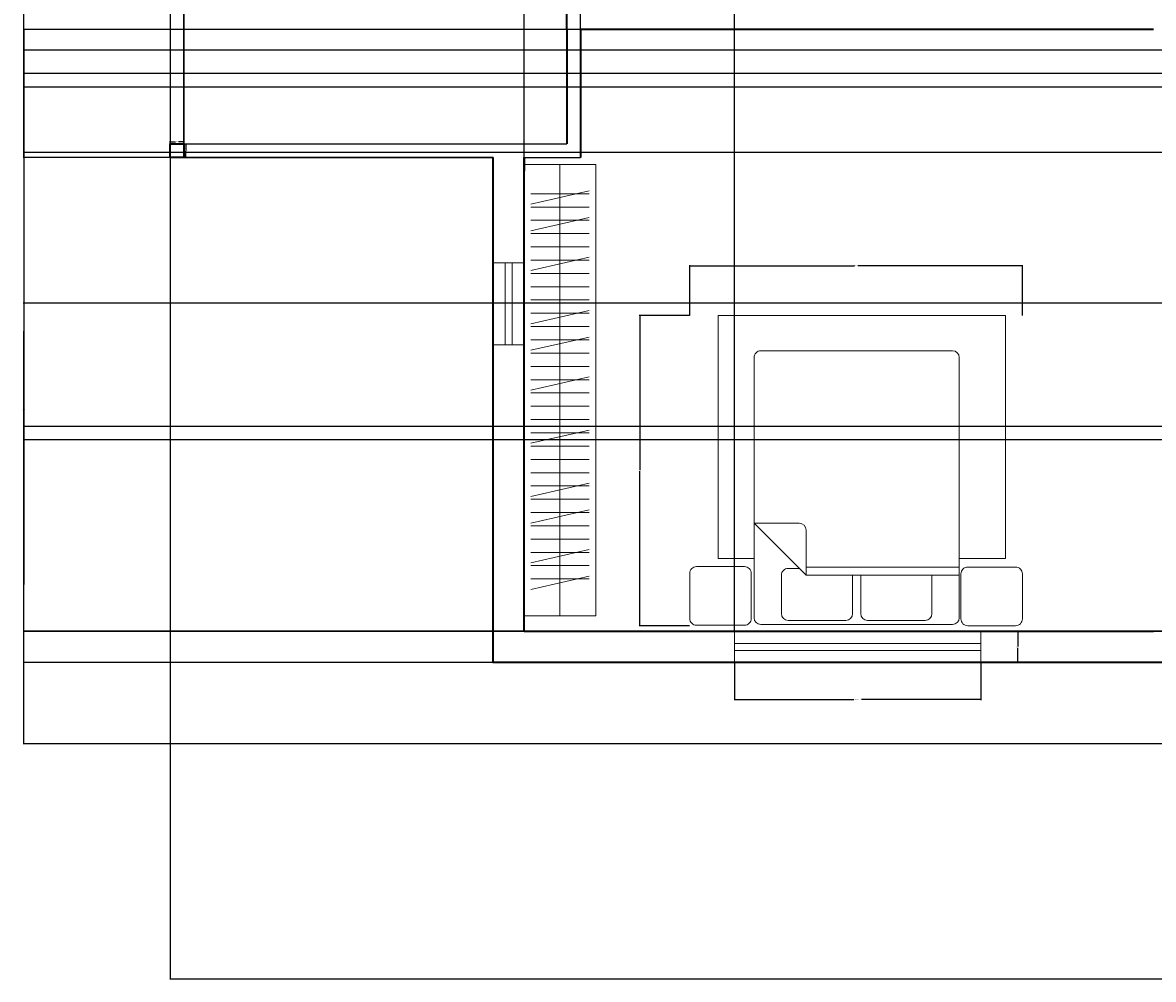
# Model space of a CAD drawing. Units: inches. Extents: x 2024 to 2965, y 1692 to 2308.
# Tile 1 of 8: x 2024 to 2355, y 1692 to 1972. Entities that reach past the tile are written whole.
import ezdxf

# ---------------------------------------------------------------- set-up
doc = ezdxf.new("R2010")
doc.units = ezdxf.units.IN
for name, color, linetype, lineweight in [('A-ANNO-DIMS', 2, 'Continuous', 18), ('A-COLS', 1, 'Continuous', 35), ('A-FLOR-CASE', 33, 'Continuous', 20), ('A-FLOR-CASE-PATT', 252, 'Continuous', 13), ('A-FLOR-OTLN', 7, 'Continuous', 25), ('A-FURN', 8, 'Continuous', 18), ('A-GLAZ', 4, 'Continuous', 18), ('A-WALL', 7, 'Continuous', 35)]:
    doc.layers.add(name, color=color, linetype=linetype, lineweight=lineweight)
doc.styles.get("Standard").update_dxf_attribs({"font": 'arial.ttf'})
doc.dimstyles.get("Standard").update_dxf_attribs({"dimtxt": 0.18, "dimasz": 0.18, "dimexe": 0.18, "dimexo": 0.0625, "dimgap": 0.09, "dimtad": 0, "dimtih": 1, "dimtoh": 1, "dimdec": 4, "dimzin": 0, "dimdsep": 46, "dimtxsty": 'Standard', "dimcen": 0.09, "dimadec": 0, "dimazin": 0, "dimtfac": 1, "dimtdec": 4, "dimtofl": 0, "dimtmove": 0, "dimatfit": 3, "dimfxl": 1, "dimtolj": 1, "dimtzin": 0, "dimarcsym": 0})

# ---------------------------------------------------------------- blocks, each defined once
blk = doc.blocks.new('Bed - Queen')
for p, q in [((2, 0), (58, 0)), ((0, -78), (0, -2)), ((8, -14.4), (8, -3.2)), ((10, -1.2), (26.8, -1.2)), ((28.8, -3.2), (28.8, -14.4)), ((31.2, -14.4), (31.2, -3.2)), ((33.2, -1.2), (50, -1.2)), ((52, -3.2), (52, -14.4)), ((60, -2), (60, -78)), ((0, -14.4), (44.8, -14.4)), ((60, -29.6), (44.8, -14.4)), ((44.8, -14.4), (44.8, -27.6)), ((50, -16.4), (46.8, -16.4)), ((44.8, -16.8), (0, -16.8)), ((46.8, -29.6), (60, -29.6)), ((58, -80), (2, -80))]:
    blk.add_line(p, q)
for points in [[(-16.47, 0.34), (-2.47, 0.34, -0.414214), (-0.47, -1.66), (-0.47, -14.8, -0.414214), (-2.47, -16.8), (-16.47, -16.8, -0.414214), (-18.47, -14.8), (-18.47, -1.66, -0.414214)], [(62.82, 0.21), (76.82, 0.21, -0.414214), (78.82, -1.79), (78.82, -14.93, -0.414214), (76.82, -16.93), (62.82, -16.93, -0.414214), (60.82, -14.93), (60.82, -1.79, -0.414214)]]:
    blk.add_lwpolyline(points, format="xyb", close=True)
blk.add_lwpolyline([(0, -19.29), (-13.55, -19.29), (-13.55, -90.28), (70.45, -90.28), (70.45, -19.29), (60, -19.29)])
for centre, start, end in [((2, -2), 90, 180), ((58, -2), 0, 90), ((10, -3.2), 90, 180), ((26.8, -3.2), 0, 90), ((33.2, -3.2), 90, 180), ((50, -3.2), 0, 90), ((50, -14.4), 270, 0), ((46.8, -27.6), 180, 270), ((2, -78), 180, 270), ((58, -78), 270, 0)]:
    blk.add_arc(centre, 2, start, end)
blk = doc.blocks.new('WIN-24-D9')
for p, q in [((0, 5.5), (24, 5.5)), ((0, 3.5), (24, 3.5))]:
    blk.add_line(p, q)
for points in [[(0, 0), (0, 9)], [(24, 9), (24, 0)]]:
    blk.add_lwpolyline(points)
blk = doc.blocks.new('WIN-72-D9')
for p, q in [((0, 5.5), (72, 5.5)), ((0, 3.5), (72, 3.5))]:
    blk.add_line(p, q)
for points in [[(0, 0), (0, 9)], [(72, 9), (72, 0)]]:
    blk.add_lwpolyline(points)
blk = doc.blocks.new('POST-4X4')
blk.add_lwpolyline([(0, 4), (4, 4), (4, 0), (0, 0)], close=True)
blk = doc.blocks.new('*D33')
at = {"layer": 'A-ANNO-DIMS', "color": 0, "lineweight": -2, "transparency": 16777216}
for p, q in [((2232.43, 1784.71), (2232.43, 1773.79)), ((2304.43, 1784.71), (2304.43, 1773.79)), ((2232.61, 1773.97), (2267.31, 1773.97)), ((2304.25, 1773.97), (2269.55, 1773.97))]:
    blk.add_line(p, q, dxfattribs=at)
at = {"layer": 'A-ANNO-DIMS', "color": 0, "transparency": 16777216}
for points in [[(2232.61, 1774), (2232.61, 1773.94), (2232.43, 1773.97)], [(2304.25, 1774), (2304.25, 1773.94), (2304.43, 1773.97)]]:
    blk.add_solid(points, dxfattribs=at)
at = {"layer": 'Defpoints', "color": 0, "transparency": 16777216}
for p in [(2232.43, 1784.77), (2304.43, 1784.77), (2304.43, 1773.97)]:
    blk.add_point(p, dxfattribs=at)
at = {"layer": 'A-ANNO-DIMS', "color": 0, "transparency": 16777216, "insert": (2268.43, 1773.97), "char_height": 0.18, "attachment_point": 5}
blk.add_mtext('\\A1;WINDOW 72 TYP.', dxfattribs=at)
blk = doc.blocks.new('*D34')
at = {"layer": 'A-ANNO-DIMS', "color": 0, "lineweight": -2, "transparency": 16777216}
for p, q in [((2304.49, 1793.77), (2315.41, 1793.77)), ((2315.23, 1793.59), (2315.23, 1789.46)), ((2315.23, 1784.95), (2315.23, 1789.09)), ((2304.49, 1784.77), (2315.41, 1784.77))]:
    blk.add_line(p, q, dxfattribs=at)
at = {"layer": 'A-ANNO-DIMS', "color": 0, "transparency": 16777216}
for points in [[(2315.2, 1793.59), (2315.26, 1793.59), (2315.23, 1793.77)], [(2315.2, 1784.95), (2315.26, 1784.95), (2315.23, 1784.77)]]:
    blk.add_solid(points, dxfattribs=at)
at = {"layer": 'Defpoints', "color": 0, "transparency": 16777216}
for p in [(2304.43, 1793.77), (2315.23, 1793.77), (2304.43, 1784.77)]:
    blk.add_point(p, dxfattribs=at)
at = {"layer": 'A-ANNO-DIMS', "color": 0, "transparency": 16777216, "insert": (2315.23, 1789.27), "char_height": 0.18, "attachment_point": 5}
blk.add_mtext('\\A1;9 TYP.', dxfattribs=at)
blk = doc.blocks.new('*D45')
at = {"layer": 'A-ANNO-DIMS', "color": 0, "lineweight": -2, "transparency": 16777216}
for p, q in [((2219.34, 1886.2), (2219.34, 1900.91)), ((2219.52, 1900.73), (2267.48, 1900.73)), ((2316.45, 1900.73), (2268.49, 1900.73)), ((2316.63, 1886.2), (2316.63, 1900.91))]:
    blk.add_line(p, q, dxfattribs=at)
at = {"layer": 'A-ANNO-DIMS', "color": 0, "transparency": 16777216}
for points in [[(2219.52, 1900.76), (2219.52, 1900.7), (2219.34, 1900.73)], [(2316.45, 1900.76), (2316.45, 1900.7), (2316.63, 1900.73)]]:
    blk.add_solid(points, dxfattribs=at)
at = {"layer": 'Defpoints', "color": 0, "transparency": 16777216}
for p in [(2219.34, 1900.73), (2219.34, 1886.14), (2316.63, 1886.14)]:
    blk.add_point(p, dxfattribs=at)
at = {"layer": 'A-ANNO-DIMS', "color": 0, "transparency": 16777216, "insert": (2267.99, 1900.73), "char_height": 0.18, "attachment_point": 5}
blk.add_mtext('\\A1;BED 97', dxfattribs=at)
blk = doc.blocks.new('*D46')
at = {"layer": 'A-ANNO-DIMS', "color": 0, "lineweight": -2, "transparency": 16777216}
for p, q in [((2219.27, 1886.14), (2204.56, 1886.14)), ((2204.74, 1885.96), (2204.74, 1841.01)), ((2204.74, 1795.7), (2204.74, 1840.65)), ((2219.27, 1795.52), (2204.56, 1795.52))]:
    blk.add_line(p, q, dxfattribs=at)
at = {"layer": 'A-ANNO-DIMS', "color": 0, "transparency": 16777216}
for points in [[(2204.71, 1885.96), (2204.77, 1885.96), (2204.74, 1886.14)], [(2204.71, 1795.7), (2204.77, 1795.7), (2204.74, 1795.52)]]:
    blk.add_solid(points, dxfattribs=at)
at = {"layer": 'Defpoints', "color": 0, "transparency": 16777216}
for p in [(2219.34, 1886.14), (2204.74, 1795.52), (2219.34, 1795.52)]:
    blk.add_point(p, dxfattribs=at)
at = {"layer": 'A-ANNO-DIMS', "color": 0, "transparency": 16777216, "insert": (2204.74, 1840.83), "char_height": 0.18, "attachment_point": 5}
blk.add_mtext('\\A1;91', dxfattribs=at)
blk = doc.blocks.new('*D55')
at = {"layer": 'A-ANNO-DIMS', "color": 0, "lineweight": -2, "transparency": 16777216}
for p, q in [((2071.52, 1936.35), (2072.24, 1936.35)), ((2072.06, 1936.17), (2072.06, 1934.54)), ((2072.06, 1932.53), (2072.06, 1934.17)), ((2071.52, 1932.35), (2072.24, 1932.35))]:
    blk.add_line(p, q, dxfattribs=at)
at = {"layer": 'A-ANNO-DIMS', "color": 0, "transparency": 16777216}
for points in [[(2072.03, 1936.17), (2072.09, 1936.17), (2072.06, 1936.35)], [(2072.03, 1932.53), (2072.09, 1932.53), (2072.06, 1932.35)]]:
    blk.add_solid(points, dxfattribs=at)
at = {"layer": 'Defpoints', "color": 0, "transparency": 16777216}
for p in [(2071.46, 1936.35), (2072.06, 1936.35), (2071.46, 1932.35)]:
    blk.add_point(p, dxfattribs=at)
at = {"layer": 'A-ANNO-DIMS', "color": 0, "transparency": 16777216, "insert": (2072.06, 1934.35), "char_height": 0.18, "attachment_point": 5}
blk.add_mtext('\\A1;POST 4 TYP.', dxfattribs=at)
blk = doc.blocks.new('*D56')
at = {"layer": 'A-ANNO-DIMS', "color": 0, "lineweight": -2, "transparency": 16777216}
for p, q in [((2067.46, 1936.41), (2067.46, 1937.13)), ((2067.64, 1936.95), (2069, 1936.95)), ((2071.28, 1936.95), (2069.92, 1936.95)), ((2071.46, 1936.41), (2071.46, 1937.13))]:
    blk.add_line(p, q, dxfattribs=at)
at = {"layer": 'A-ANNO-DIMS', "color": 0, "transparency": 16777216}
for points in [[(2067.64, 1936.98), (2067.64, 1936.92), (2067.46, 1936.95)], [(2071.28, 1936.98), (2071.28, 1936.92), (2071.46, 1936.95)]]:
    blk.add_solid(points, dxfattribs=at)
at = {"layer": 'Defpoints', "color": 0, "transparency": 16777216}
for p in [(2067.46, 1936.95), (2067.46, 1936.35), (2071.46, 1936.35)]:
    blk.add_point(p, dxfattribs=at)
at = {"layer": 'A-ANNO-DIMS', "color": 0, "transparency": 16777216, "insert": (2069.46, 1936.95), "char_height": 0.18, "attachment_point": 5}
blk.add_mtext('\\A1;4 TYP.', dxfattribs=at)
blk = doc.blocks.new('*D75')
at = {"layer": 'A-ANNO-DIMS', "color": 0, "lineweight": -2, "transparency": 16777216}
for p, q in [((2922.02, 1952.85), (2922.02, 1692.14)), ((2067.46, 1932.29), (2067.46, 1692.14)), ((2067.64, 1692.32), (2494.35, 1692.32)), ((2921.84, 1692.32), (2495.13, 1692.32))]:
    blk.add_line(p, q, dxfattribs=at)
at = {"layer": 'A-ANNO-DIMS', "color": 0, "transparency": 16777216}
for points in [[(2067.64, 1692.35), (2067.64, 1692.29), (2067.46, 1692.32)], [(2921.84, 1692.35), (2921.84, 1692.29), (2922.02, 1692.32)]]:
    blk.add_solid(points, dxfattribs=at)
at = {"layer": 'Defpoints', "color": 0, "transparency": 16777216}
for p in [(2922.02, 1952.91), (2067.46, 1932.35), (2922.02, 1692.32)]:
    blk.add_point(p, dxfattribs=at)
at = {"layer": 'A-ANNO-DIMS', "color": 0, "transparency": 16777216, "insert": (2494.74, 1692.32), "char_height": 0.18, "attachment_point": 5}
blk.add_mtext('\\A1;854.6', dxfattribs=at)
blk = doc.blocks.new('*D90')
at = {"layer": 'A-ANNO-DIMS', "color": 0, "lineweight": -2, "transparency": 16777216}
for p, q in [((2067.4, 2148.35), (2024.5, 2148.35)), ((2024.68, 2148.17), (2024.68, 2040.53)), ((2024.68, 1932.53), (2024.68, 2040.17)), ((2067.4, 1932.35), (2024.5, 1932.35))]:
    blk.add_line(p, q, dxfattribs=at)
at = {"layer": 'A-ANNO-DIMS', "color": 0, "transparency": 16777216}
for points in [[(2024.65, 2148.17), (2024.71, 2148.17), (2024.68, 2148.35)], [(2024.65, 1932.53), (2024.71, 1932.53), (2024.68, 1932.35)]]:
    blk.add_solid(points, dxfattribs=at)
at = {"layer": 'Defpoints', "color": 0, "transparency": 16777216}
for p in [(2024.68, 2148.35), (2067.46, 2148.35), (2067.46, 1932.35)]:
    blk.add_point(p, dxfattribs=at)
at = {"layer": 'A-ANNO-DIMS', "color": 0, "transparency": 16777216, "insert": (2024.68, 2040.35), "char_height": 0.18, "attachment_point": 5}
blk.add_mtext('\\A1;216', dxfattribs=at)
blk = doc.blocks.new('*D91')
at = {"layer": 'A-ANNO-DIMS', "color": 0, "lineweight": -2, "transparency": 16777216}
for p, q in [((2071.46, 1936.41), (2071.46, 2307.73)), ((2183.46, 1936.41), (2183.46, 2307.73)), ((2071.64, 2307.55), (2127.18, 2307.55)), ((2183.28, 2307.55), (2127.74, 2307.55))]:
    blk.add_line(p, q, dxfattribs=at)
at = {"layer": 'A-ANNO-DIMS', "color": 0, "transparency": 16777216}
for points in [[(2071.64, 2307.58), (2071.64, 2307.52), (2071.46, 2307.55)], [(2183.28, 2307.58), (2183.28, 2307.52), (2183.46, 2307.55)]]:
    blk.add_solid(points, dxfattribs=at)
at = {"layer": 'Defpoints', "color": 0, "transparency": 16777216}
for p in [(2183.46, 2307.55), (2071.46, 1936.35), (2183.46, 1936.35)]:
    blk.add_point(p, dxfattribs=at)
at = {"layer": 'A-ANNO-DIMS', "color": 0, "transparency": 16777216, "insert": (2127.46, 2307.55), "char_height": 0.18, "attachment_point": 5}
blk.add_mtext('\\A1;112', dxfattribs=at)
blk = doc.blocks.new('*D92')
at = {"layer": 'A-ANNO-DIMS', "color": 0, "lineweight": -2, "transparency": 16777216}
for p, q in [((2187.4, 1969.77), (2024.5, 1969.77)), ((2024.68, 1969.59), (2024.68, 1881.96)), ((2024.68, 1793.95), (2024.68, 1881.59)), ((2170.84, 1793.77), (2024.5, 1793.77))]:
    blk.add_line(p, q, dxfattribs=at)
at = {"layer": 'A-ANNO-DIMS', "color": 0, "transparency": 16777216}
for points in [[(2024.65, 1969.59), (2024.71, 1969.59), (2024.68, 1969.77)], [(2024.65, 1793.95), (2024.71, 1793.95), (2024.68, 1793.77)]]:
    blk.add_solid(points, dxfattribs=at)
at = {"layer": 'Defpoints', "color": 0, "transparency": 16777216}
for p in [(2024.68, 1969.77), (2187.46, 1969.77), (2170.91, 1793.77)]:
    blk.add_point(p, dxfattribs=at)
at = {"layer": 'A-ANNO-DIMS', "color": 0, "transparency": 16777216, "insert": (2024.68, 1881.77), "char_height": 0.18, "attachment_point": 5}
blk.add_mtext('\\A1;176', dxfattribs=at)
blk = doc.blocks.new('*D93')
at = {"layer": 'A-ANNO-DIMS', "color": 0, "lineweight": -2, "transparency": 16777216}
for p, q in [((2187.46, 1932.41), (2187.46, 2307.73)), ((2418.91, 1933.84), (2418.91, 2307.73)), ((2187.64, 2307.55), (2302.72, 2307.55)), ((2418.73, 2307.55), (2303.65, 2307.55))]:
    blk.add_line(p, q, dxfattribs=at)
at = {"layer": 'A-ANNO-DIMS', "color": 0, "transparency": 16777216}
for points in [[(2187.64, 2307.58), (2187.64, 2307.52), (2187.46, 2307.55)], [(2418.73, 2307.58), (2418.73, 2307.52), (2418.91, 2307.55)]]:
    blk.add_solid(points, dxfattribs=at)
at = {"layer": 'Defpoints', "color": 0, "transparency": 16777216}
for p in [(2418.91, 2307.55), (2187.46, 1932.35), (2418.91, 1933.77)]:
    blk.add_point(p, dxfattribs=at)
at = {"layer": 'A-ANNO-DIMS', "color": 0, "transparency": 16777216, "insert": (2303.18, 2307.55), "char_height": 0.18, "attachment_point": 5}
blk.add_mtext('\\A1;231.45', dxfattribs=at)
blk = doc.blocks.new('*D97')
at = {"layer": 'A-ANNO-DIMS', "color": 0, "lineweight": -2, "transparency": 16777216}
for p, q in [((2358.84, 1889.77), (2024.5, 1889.77)), ((2024.68, 1889.59), (2024.68, 1841.96)), ((2024.68, 1793.95), (2024.68, 1841.59)), ((2358.84, 1793.77), (2024.5, 1793.77))]:
    blk.add_line(p, q, dxfattribs=at)
at = {"layer": 'A-ANNO-DIMS', "color": 0, "transparency": 16777216}
for points in [[(2024.65, 1889.59), (2024.71, 1889.59), (2024.68, 1889.77)], [(2024.65, 1793.95), (2024.71, 1793.95), (2024.68, 1793.77)]]:
    blk.add_solid(points, dxfattribs=at)
at = {"layer": 'Defpoints', "color": 0, "transparency": 16777216}
for p in [(2358.91, 1889.77), (2024.68, 1793.77), (2358.91, 1793.77)]:
    blk.add_point(p, dxfattribs=at)
at = {"layer": 'A-ANNO-DIMS', "color": 0, "transparency": 16777216, "insert": (2024.68, 1841.77), "char_height": 0.18, "attachment_point": 5}
blk.add_mtext('\\A1;96', dxfattribs=at)
blk = doc.blocks.new('*D101')
at = {"layer": 'A-ANNO-DIMS', "color": 0, "lineweight": -2, "transparency": 16777216}
for p, q in [((2917.96, 2113.77), (2024.5, 2113.77)), ((2024.68, 2113.59), (2024.68, 2035.52)), ((2024.68, 1957.09), (2024.68, 2035.16)), ((2917.96, 1956.91), (2024.5, 1956.91))]:
    blk.add_line(p, q, dxfattribs=at)
at = {"layer": 'A-ANNO-DIMS', "color": 0, "transparency": 16777216}
for points in [[(2024.65, 2113.59), (2024.71, 2113.59), (2024.68, 2113.77)], [(2024.65, 1957.09), (2024.71, 1957.09), (2024.68, 1956.91)]]:
    blk.add_solid(points, dxfattribs=at)
at = {"layer": 'Defpoints', "color": 0, "transparency": 16777216}
for p in [(2024.68, 2113.77), (2918.02, 2113.77), (2918.02, 1956.91)]:
    blk.add_point(p, dxfattribs=at)
at = {"layer": 'A-ANNO-DIMS', "color": 0, "transparency": 16777216, "insert": (2024.68, 2035.34), "char_height": 0.18, "attachment_point": 5}
blk.add_mtext('\\A1;156.87', dxfattribs=at)
blk = doc.blocks.new('*D102')
at = {"layer": 'A-ANNO-DIMS', "color": 0, "lineweight": -2, "transparency": 16777216}
for p, q in [((2830.9, 1952.91), (2024.5, 1952.91)), ((2024.68, 1952.73), (2024.68, 1873.58)), ((2024.68, 1794.07), (2024.68, 1873.22)), ((2830.9, 1793.89), (2024.5, 1793.89))]:
    blk.add_line(p, q, dxfattribs=at)
at = {"layer": 'A-ANNO-DIMS', "color": 0, "transparency": 16777216}
for points in [[(2024.65, 1952.73), (2024.71, 1952.73), (2024.68, 1952.91)], [(2024.65, 1794.07), (2024.71, 1794.07), (2024.68, 1793.89)]]:
    blk.add_solid(points, dxfattribs=at)
at = {"layer": 'Defpoints', "color": 0, "transparency": 16777216}
for p in [(2830.96, 1952.91), (2024.68, 1793.89), (2830.96, 1793.89)]:
    blk.add_point(p, dxfattribs=at)
at = {"layer": 'A-ANNO-DIMS', "color": 0, "transparency": 16777216, "insert": (2024.68, 1873.4), "char_height": 0.18, "attachment_point": 5}
blk.add_mtext('\\A1;159', dxfattribs=at)
blk = doc.blocks.new('*D104')
at = {"layer": 'A-ANNO-DIMS', "color": 0, "lineweight": -2, "transparency": 16777216}
for p, q in [((2418.84, 1963.77), (2024.5, 1963.77)), ((2024.68, 1963.59), (2024.68, 1948.96)), ((2024.68, 1933.95), (2024.68, 1948.59)), ((2418.84, 1933.77), (2024.5, 1933.77))]:
    blk.add_line(p, q, dxfattribs=at)
at = {"layer": 'A-ANNO-DIMS', "color": 0, "transparency": 16777216}
for points in [[(2024.65, 1963.59), (2024.71, 1963.59), (2024.68, 1963.77)], [(2024.65, 1933.95), (2024.71, 1933.95), (2024.68, 1933.77)]]:
    blk.add_solid(points, dxfattribs=at)
at = {"layer": 'Defpoints', "color": 0, "transparency": 16777216}
for p in [(2418.91, 1963.77), (2024.68, 1933.77), (2418.91, 1933.77)]:
    blk.add_point(p, dxfattribs=at)
at = {"layer": 'A-ANNO-DIMS', "color": 0, "transparency": 16777216, "insert": (2024.68, 1948.77), "char_height": 0.18, "attachment_point": 5}
blk.add_mtext('\\A1;30', dxfattribs=at)
blk = doc.blocks.new('*D111')
at = {"layer": 'A-ANNO-DIMS', "color": 0, "lineweight": -2, "transparency": 16777216}
for p, q in [((2668.84, 1849.79), (2024.5, 1849.79)), ((2024.68, 1849.61), (2024.68, 1821.96)), ((2024.68, 1793.95), (2024.68, 1821.6)), ((2668.84, 1793.77), (2024.5, 1793.77))]:
    blk.add_line(p, q, dxfattribs=at)
at = {"layer": 'A-ANNO-DIMS', "color": 0, "transparency": 16777216}
for points in [[(2024.65, 1849.61), (2024.71, 1849.61), (2024.68, 1849.79)], [(2024.65, 1793.95), (2024.71, 1793.95), (2024.68, 1793.77)]]:
    blk.add_solid(points, dxfattribs=at)
at = {"layer": 'Defpoints', "color": 0, "transparency": 16777216}
for p in [(2024.68, 1849.79), (2668.91, 1849.79), (2668.91, 1793.77)]:
    blk.add_point(p, dxfattribs=at)
at = {"layer": 'A-ANNO-DIMS', "color": 0, "transparency": 16777216, "insert": (2024.68, 1821.78), "char_height": 0.18, "attachment_point": 5}
blk.add_mtext('\\A1;56.01', dxfattribs=at)
blk = doc.blocks.new('*D113')
at = {"layer": 'A-ANNO-DIMS', "color": 0, "lineweight": -2, "transparency": 16777216}
for p, q in [((2161.84, 1932.35), (2024.5, 1932.35)), ((2024.68, 1932.17), (2024.68, 1858.74)), ((2024.68, 1784.95), (2024.68, 1858.38)), ((2161.84, 1784.77), (2024.5, 1784.77))]:
    blk.add_line(p, q, dxfattribs=at)
at = {"layer": 'A-ANNO-DIMS', "color": 0, "transparency": 16777216}
for points in [[(2024.65, 1932.17), (2024.71, 1932.17), (2024.68, 1932.35)], [(2024.65, 1784.95), (2024.71, 1784.95), (2024.68, 1784.77)]]:
    blk.add_solid(points, dxfattribs=at)
at = {"layer": 'Defpoints', "color": 0, "transparency": 16777216}
for p in [(2161.91, 1932.35), (2024.68, 1784.77), (2161.91, 1784.77)]:
    blk.add_point(p, dxfattribs=at)
at = {"layer": 'A-ANNO-DIMS', "color": 0, "transparency": 16777216, "insert": (2024.68, 1858.56), "char_height": 0.18, "attachment_point": 5}
blk.add_mtext('\\A1;147.58', dxfattribs=at)
blk = doc.blocks.new('*D115')
at = {"layer": 'A-ANNO-DIMS', "color": 0, "lineweight": -2, "transparency": 16777216}
for p, q in [((2548.84, 1853.77), (2024.5, 1853.77)), ((2024.68, 1853.59), (2024.68, 1807.54)), ((2024.68, 1761.13), (2024.68, 1807.18)), ((2548.84, 1760.95), (2024.5, 1760.95))]:
    blk.add_line(p, q, dxfattribs=at)
at = {"layer": 'A-ANNO-DIMS', "color": 0, "transparency": 16777216}
for points in [[(2024.65, 1853.59), (2024.71, 1853.59), (2024.68, 1853.77)], [(2024.65, 1761.13), (2024.71, 1761.13), (2024.68, 1760.95)]]:
    blk.add_solid(points, dxfattribs=at)
at = {"layer": 'Defpoints', "color": 0, "transparency": 16777216}
for p in [(2024.68, 1853.77), (2548.91, 1853.77), (2548.91, 1760.95)]:
    blk.add_point(p, dxfattribs=at)
at = {"layer": 'A-ANNO-DIMS', "color": 0, "transparency": 16777216, "insert": (2024.68, 1807.36), "char_height": 0.18, "attachment_point": 5}
blk.add_mtext('\\A1;92.82', dxfattribs=at)
blk = doc.blocks.new('*D116')
at = {"layer": 'A-ANNO-DIMS', "color": 0, "lineweight": -2, "transparency": 16777216}
for p, q in [((2170.91, 1793.84), (2170.91, 2307.73)), ((2232.43, 1793.84), (2232.43, 2307.73)), ((2171.09, 2307.55), (2201.27, 2307.55)), ((2232.25, 2307.55), (2202.06, 2307.55))]:
    blk.add_line(p, q, dxfattribs=at)
at = {"layer": 'A-ANNO-DIMS', "color": 0, "transparency": 16777216}
for points in [[(2171.09, 2307.58), (2171.09, 2307.52), (2170.91, 2307.55)], [(2232.25, 2307.58), (2232.25, 2307.52), (2232.43, 2307.55)]]:
    blk.add_solid(points, dxfattribs=at)
at = {"layer": 'Defpoints', "color": 0, "transparency": 16777216}
for p in [(2232.43, 2307.55), (2170.91, 1793.77), (2232.43, 1793.77)]:
    blk.add_point(p, dxfattribs=at)
at = {"layer": 'A-ANNO-DIMS', "color": 0, "transparency": 16777216, "insert": (2201.67, 2307.55), "char_height": 0.18, "attachment_point": 5}
blk.add_mtext('\\A1;61.52', dxfattribs=at)

msp = doc.modelspace()

# ---------------------------------------------------------------- hatches: boundary and pattern name
at = {"layer": 'A-FLOR-CASE-PATT'}
h = msp.add_hatch(dxfattribs=at)
h.set_pattern_fill('ANSI31', color=256, scale=1.222788, angle=-45, style=0)
h.paths.add_polyline_path([(2172.9061, 1806.1167), (2189.9061, 1806.1167), (2189.9061, 1922.5873), (2172.9061, 1922.5873)])

# ---------------------------------------------------------------- linework, layer by layer
at = {"layer": 'A-FLOR-CASE'}
for p, q in [((2191.9061, 1930.352), (2170.9061, 1930.352)), ((2170.9061, 1930.352), (2170.9061, 1798.352)), ((2181.4061, 1930.352), (2181.4061, 1798.352)), ((2191.9061, 1798.352), (2191.9061, 1930.352)), ((2170.9061, 1798.352), (2191.9061, 1798.352)), ((2191.9061, 1798.352), (2170.9061, 1798.352))]:
    msp.add_line(p, q, dxfattribs=at)
at = {"layer": 'A-FLOR-CASE-PATT'}
for p, q in [((2189.9061, 1922.5873), (2172.9061, 1918.7049)), ((2189.9061, 1914.8226), (2172.9061, 1910.9402)), ((2189.9061, 1903.1755), (2172.9061, 1899.2932)), ((2189.9061, 1887.6461), (2172.9061, 1883.7638)), ((2189.9061, 1879.8814), (2172.9061, 1875.999)), ((2189.9061, 1868.2343), (2172.9061, 1864.352)), ((2189.9061, 1852.7049), (2172.9061, 1848.8226)), ((2189.9061, 1837.1755), (2172.9061, 1833.2932)), ((2189.9061, 1829.4108), (2172.9061, 1825.5285)), ((2189.9061, 1817.7638), (2172.9061, 1813.8814)), ((2189.9061, 1809.999), (2172.9061, 1806.1167))]:
    msp.add_line(p, q, dxfattribs=at)
at = {"layer": 'A-FLOR-OTLN'}
for p, q in [((2170.9061, 1936.352), (2183.4594, 1936.352)), ((2170.9061, 1932.352), (2187.4594, 1932.352))]:
    msp.add_line(p, q, dxfattribs=at)
for points in [[(2161.9061, 2148.352), (2067.4594, 2148.352), (2067.4594, 1932.352), (2161.9061, 1932.352)], [(2161.9061, 2144.352), (2071.4594, 2144.352), (2071.4594, 1936.352), (2170.9061, 1936.352)]]:
    msp.add_lwpolyline(points, dxfattribs=at)
at = {"layer": 'A-WALL'}
for p, q in [((2183.4594, 1969.7736), (2183.4594, 1936.352)), ((2187.4594, 1969.7736), (2187.4594, 1932.352)), ((2354.9061, 1969.7736), (2187.4594, 1969.7736)), ((2170.9061, 1793.7736), (2170.9061, 1932.352)), ((2170.9061, 1932.352), (2170.9061, 1928.352)), ((2354.9061, 1793.7736), (2170.9061, 1793.7736))]:
    msp.add_line(p, q, dxfattribs=at)
for points in [[(2183.4594, 1969.7736), (2183.4594, 2131.7736)], [(2422.9061, 1784.7736), (2161.9061, 1784.7736), (2161.9061, 1932.352)]]:
    msp.add_lwpolyline(points, dxfattribs=at)

# ---------------------------------------------------------------- block references
at = {"layer": 'A-COLS', "rotation": 90}
msp.add_blockref('POST-4X4', (2071.4594, 1932.3516), dxfattribs=at)
at = {"layer": 'A-FURN', "rotation": 180}
msp.add_blockref('Bed - Queen', (2298.1595, 1795.8593), dxfattribs=at)
at = {"layer": 'A-GLAZ', "rotation": 270.0000000000003}
msp.add_blockref('WIN-24-D9', (2161.9065, 1901.6146), dxfattribs=at)
at = {"layer": 'A-GLAZ'}
msp.add_blockref('WIN-72-D9', (2232.4294, 1784.774), dxfattribs=at)

# ---------------------------------------------------------------- dimensions: what is measured, and where the dimension line sits
at = {"layer": 'A-ANNO-DIMS'}
for base, p1, p2, override, picture, middle in [((2183.4594, 2307.5486), (2071.4594, 1936.352), (2183.4594, 1936.352), {"dimdec": 0, "dimlfac": 1, "dimrnd": 0, "dimzin": 0, "dimdsep": 46, "dimlunit": 2}, '*D91', (2127.4594, 2307.5486)), ((2232.4289, 2307.5486), (2170.9061, 1793.7736), (2232.4289, 1793.7736), {"dimdec": 2, "dimlfac": 1, "dimrnd": 0, "dimzin": 0, "dimdsep": 46, "dimlunit": 2}, '*D116', (2201.6675, 2307.5486)), ((2418.9061, 2307.5486), (2187.4594, 1932.352), (2418.9061, 1933.7736), {"dimdec": 2, "dimlfac": 1, "dimrnd": 0, "dimzin": 0, "dimdsep": 46, "dimlunit": 2}, '*D93', (2303.1828, 2307.5486)), ((2922.0192, 1692.3236), (2067.4594, 1932.352), (2922.0192, 1952.9082), {"dimdec": 1, "dimlfac": 1, "dimrnd": 0, "dimzin": 0, "dimdsep": 46, "dimlunit": 2}, '*D75', (2494.7393, 1692.3236))]:
    dim = msp.add_linear_dim(base=base, p1=p1, p2=p2, dimstyle='Standard', override=override, dxfattribs=at)
    dim.commit()
    dim.dimension.update_dxf_attribs({"geometry": picture, "text_midpoint": middle})
for base, p1, p2, angle, override, picture, middle in [((2024.6844, 2148.352), (2067.4594, 1932.352), (2067.4594, 2148.352), 90, {"dimdec": 0, "dimlfac": 1, "dimrnd": 0, "dimzin": 0, "dimdsep": 46, "dimlunit": 2}, '*D90', (2024.6844, 2040.352)), ((2024.6844, 2113.7736), (2918.0192, 1956.9082), (2918.0192, 2113.7736), 90, {"dimdec": 2, "dimlfac": 1, "dimrnd": 0, "dimzin": 0, "dimdsep": 46, "dimlunit": 2}, '*D101', (2024.6844, 2035.3409)), ((2024.6844, 1969.7736), (2170.9061, 1793.7736), (2187.4594, 1969.7736), 90, {"dimdec": 0, "dimlfac": 1, "dimrnd": 0, "dimzin": 0, "dimdsep": 46, "dimlunit": 2}, '*D92', (2024.6844, 1881.7736)), ((2024.6844, 1933.7736), (2418.9061, 1963.7736), (2418.9061, 1933.7736), 90, {"dimdec": 0, "dimlfac": 1, "dimrnd": 0, "dimzin": 0, "dimdsep": 46, "dimlunit": 2}, '*D104', (2024.6844, 1948.7736)), ((2024.6844, 1793.8927), (2830.9627, 1952.9082), (2830.9627, 1793.8927), 90, {"dimdec": 0, "dimlfac": 1, "dimrnd": 0, "dimzin": 0, "dimdsep": 46, "dimlunit": 2}, '*D102', (2024.6844, 1873.4004)), ((2024.6844, 1784.7736), (2161.9061, 1932.352), (2161.9061, 1784.7736), 90, {"dimdec": 2, "dimlfac": 1, "dimrnd": 0, "dimzin": 0, "dimdsep": 46, "dimlunit": 2}, '*D113', (2024.6844, 1858.5628)), ((2024.6844, 1793.7736), (2358.9061, 1889.7736), (2358.9061, 1793.7736), 90, {"dimdec": 0, "dimlfac": 1, "dimrnd": 0, "dimzin": 0, "dimdsep": 46, "dimlunit": 2}, '*D97', (2024.6844, 1841.7736)), ((2204.7427, 1795.5186), (2219.3371, 1886.1373), (2219.3371, 1795.5186), 270, {"dimdec": 0, "dimlfac": 1, "dimrnd": 0, "dimzin": 0, "dimdsep": 46, "dimlunit": 2}, '*D46', (2204.7427, 1840.828)), ((2024.6844, 1853.7736), (2548.9061, 1760.9504), (2548.9061, 1853.7736), 90, {"dimdec": 2, "dimlfac": 1, "dimrnd": 0, "dimzin": 0, "dimdsep": 46, "dimlunit": 2}, '*D115', (2024.6844, 1807.362)), ((2024.6844, 1849.7881), (2668.9061, 1793.7736), (2668.9061, 1849.7881), 90, {"dimdec": 2, "dimlfac": 1, "dimrnd": 0, "dimzin": 0, "dimdsep": 46, "dimlunit": 2}, '*D111', (2024.6844, 1821.7809))]:
    dim = msp.add_linear_dim(base=base, p1=p1, p2=p2, angle=angle, dimstyle='Standard', override=override, dxfattribs=at)
    dim.commit()
    dim.dimension.update_dxf_attribs({"geometry": picture, "text_midpoint": middle})
for base, p1, p2, angle, text, picture, middle in [((2067.4594, 1936.952), (2071.4594, 1936.352), (2067.4594, 1936.352), 180, '<> TYP.', '*D56', (2069.4594, 1936.952)), ((2072.0594, 1936.352), (2071.4594, 1932.352), (2071.4594, 1936.352), 90, 'POST <> TYP.', '*D55', (2072.0594, 1934.352)), ((2219.3371, 1900.7317), (2316.633, 1886.1373), (2219.3371, 1886.1373), 180, 'BED <>', '*D45', (2267.9851, 1900.7317)), ((2315.2289, 1793.7736), (2304.4289, 1784.7736), (2304.4289, 1793.7736), 90, '<> TYP.', '*D34', (2315.2289, 1789.2736))]:
    dim = msp.add_linear_dim(base=base, p1=p1, p2=p2, angle=angle, text=text, dimstyle='Standard', override={"dimdec": 0, "dimlfac": 1, "dimrnd": 0, "dimzin": 0, "dimdsep": 46, "dimlunit": 2}, dxfattribs=at)
    dim.commit()
    dim.dimension.update_dxf_attribs({"geometry": picture, "text_midpoint": middle})
dim = msp.add_linear_dim(base=(2304.4289, 1773.9736), p1=(2232.4289, 1784.7736), p2=(2304.4289, 1784.7736), text='WINDOW <> TYP.', dimstyle='Standard', override={"dimdec": 0, "dimlfac": 1, "dimrnd": 0, "dimzin": 0, "dimdsep": 46, "dimlunit": 2}, dxfattribs=at)
dim.commit()
dim.dimension.update_dxf_attribs({"geometry": '*D33', "text_midpoint": (2268.4289, 1773.9736)})

doc.saveas('drawing.dxf')
